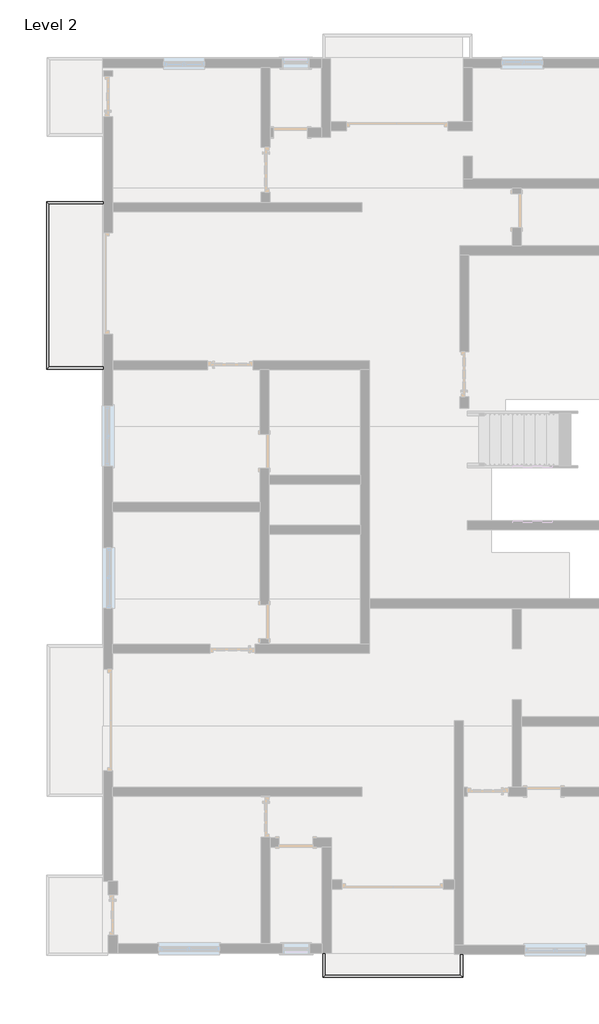
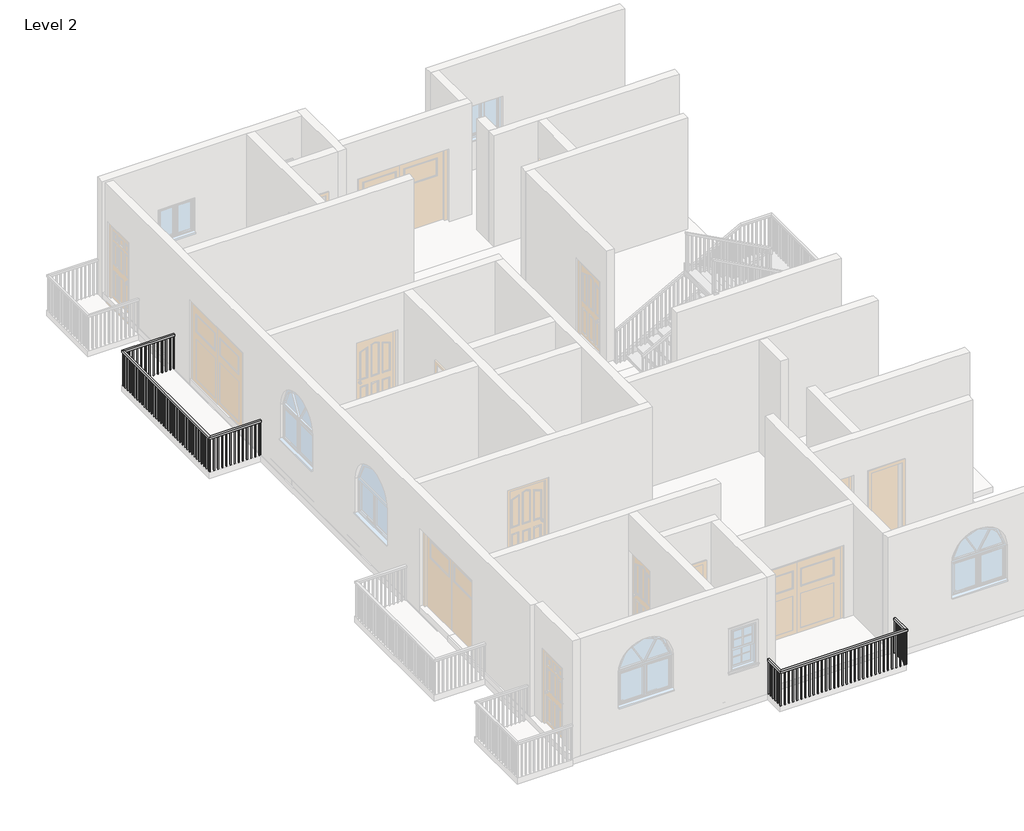
# One storey, part 4 of 7: 2 railings.
"""IFC4 building model written with IfcOpenShell, lengths in millimetres."""

from ifc_helpers import new_model, si_unit, frame, origin, place, context, project, spatial, polyline, outline, extrude, faceted_brep, element, save

model = new_model("IFC4")

# Units and contexts
model_context = context("Model", 3, world=origin())
ifc_project = project(units=[si_unit("LENGTHUNIT", "METRE", prefix="MILLI")], contexts=[model_context])

# Site, building, storey
site = spatial("IfcSite", under=ifc_project)
building = spatial("IfcBuilding", under=site)
storey = spatial("IfcBuildingStorey", under=building, Name="Level 2", Elevation=3048.0)

# Railings
placement = place(None, origin())
element("IfcRailing", 1, ObjectType="Handrail - Rectangular", at=placement, inside=storey, context=model_context, shape_type="SolidModel", body=[
    faceted_brep([(-1375.8109037, -10612.9037749, 3962.4), (-1375.8109037, -10612.9037749, 3911.6), (-1426.6109037, -10612.9037749, 3911.6), (-1426.6109037, -10612.9037749, 3962.4), (-1375.8109037, -11108.2037749, 3962.4), (-1375.8109037, -11108.2037749, 3911.6), (-1426.6109037, -11159.0037749, 3911.6), (-1426.6109037, -11159.0037749, 3962.4), (1659.4890963, -11108.2037749, 3962.4), (1659.4890963, -11108.2037749, 3911.6), (1710.2890963, -11159.0037749, 3911.6), (1710.2890963, -11159.0037749, 3962.4), (1659.4890963, -10638.3037749, 3962.4), (1710.2890963, -10638.3037749, 3962.4), (1710.2890963, -10638.3037749, 3911.6), (1659.4890963, -10638.3037749, 3911.6)], [[[0, 1, 2, 3]], [[1, 0, 4, 5]], [[2, 1, 5, 6]], [[3, 2, 6, 7]], [[0, 3, 7, 4]], [[5, 4, 8, 9]], [[6, 5, 9, 10]], [[7, 6, 10, 11]], [[4, 7, 11, 8]], [[12, 13, 14, 15]], [[9, 8, 12, 15]], [[10, 9, 15, 14]], [[11, 10, 14, 13]], [[8, 11, 13, 12]]]),
    extrude(outline(polyline([(1694.4140963, -10736.7287749), (1675.3640963, -10736.7287749), (1675.3640963, -10717.6787749), (1694.4140963, -10717.6787749), (1694.4140963, -10736.7287749)])), frame((0.0, 0.0, 3048.0), z_axis=(0.0, 0.0, 1.0), x_axis=(1.0, 0.0, 0.0)), (0.0, 0.0, 1.0), 863.6),
    extrude(outline(polyline([(1694.4140963, -10838.3287749), (1675.3640963, -10838.3287749), (1675.3640963, -10819.2787749), (1694.4140963, -10819.2787749), (1694.4140963, -10838.3287749)])), frame((0.0, 0.0, 3048.0), z_axis=(0.0, 0.0, 1.0), x_axis=(1.0, 0.0, 0.0)), (0.0, 0.0, 1.0), 863.6),
    extrude(outline(polyline([(1694.4140963, -10939.9287749), (1675.3640963, -10939.9287749), (1675.3640963, -10920.8787749), (1694.4140963, -10920.8787749), (1694.4140963, -10939.9287749)])), frame((0.0, 0.0, 3048.0), z_axis=(0.0, 0.0, 1.0), x_axis=(1.0, 0.0, 0.0)), (0.0, 0.0, 1.0), 863.6),
    extrude(outline(polyline([(1694.4140963, -11041.5287749), (1675.3640963, -11041.5287749), (1675.3640963, -11022.4787749), (1694.4140963, -11022.4787749), (1694.4140963, -11041.5287749)])), frame((0.0, 0.0, 3048.0), z_axis=(0.0, 0.0, 1.0), x_axis=(1.0, 0.0, 0.0)), (0.0, 0.0, 1.0), 863.6),
    extrude(outline(polyline([(1637.2640963, -11143.1287749), (1637.2640963, -11124.0787749), (1656.3140963, -11124.0787749), (1656.3140963, -11143.1287749), (1637.2640963, -11143.1287749)])), frame((0.0, 0.0, 3048.0), z_axis=(0.0, 0.0, 1.0), x_axis=(1.0, 0.0, 0.0)), (0.0, 0.0, 1.0), 863.6),
    extrude(outline(polyline([(1535.6640963, -11143.1287749), (1535.6640963, -11124.0787749), (1554.7140963, -11124.0787749), (1554.7140963, -11143.1287749), (1535.6640963, -11143.1287749)])), frame((0.0, 0.0, 3048.0), z_axis=(0.0, 0.0, 1.0), x_axis=(1.0, 0.0, 0.0)), (0.0, 0.0, 1.0), 863.6),
    extrude(outline(polyline([(1434.0640963, -11143.1287749), (1434.0640963, -11124.0787749), (1453.1140963, -11124.0787749), (1453.1140963, -11143.1287749), (1434.0640963, -11143.1287749)])), frame((0.0, 0.0, 3048.0), z_axis=(0.0, 0.0, 1.0), x_axis=(1.0, 0.0, 0.0)), (0.0, 0.0, 1.0), 863.6),
    extrude(outline(polyline([(1332.4640963, -11143.1287749), (1332.4640963, -11124.0787749), (1351.5140963, -11124.0787749), (1351.5140963, -11143.1287749), (1332.4640963, -11143.1287749)])), frame((0.0, 0.0, 3048.0), z_axis=(0.0, 0.0, 1.0), x_axis=(1.0, 0.0, 0.0)), (0.0, 0.0, 1.0), 863.6),
    extrude(outline(polyline([(1230.8640963, -11143.1287749), (1230.8640963, -11124.0787749), (1249.9140963, -11124.0787749), (1249.9140963, -11143.1287749), (1230.8640963, -11143.1287749)])), frame((0.0, 0.0, 3048.0), z_axis=(0.0, 0.0, 1.0), x_axis=(1.0, 0.0, 0.0)), (0.0, 0.0, 1.0), 863.6),
    extrude(outline(polyline([(1129.2640963, -11143.1287749), (1129.2640963, -11124.0787749), (1148.3140963, -11124.0787749), (1148.3140963, -11143.1287749), (1129.2640963, -11143.1287749)])), frame((0.0, 0.0, 3048.0), z_axis=(0.0, 0.0, 1.0), x_axis=(1.0, 0.0, 0.0)), (0.0, 0.0, 1.0), 863.6),
    extrude(outline(polyline([(1027.6640963, -11143.1287749), (1027.6640963, -11124.0787749), (1046.7140963, -11124.0787749), (1046.7140963, -11143.1287749), (1027.6640963, -11143.1287749)])), frame((0.0, 0.0, 3048.0), z_axis=(0.0, 0.0, 1.0), x_axis=(1.0, 0.0, 0.0)), (0.0, 0.0, 1.0), 863.6),
    extrude(outline(polyline([(926.0640963, -11143.1287749), (926.0640963, -11124.0787749), (945.1140963, -11124.0787749), (945.1140963, -11143.1287749), (926.0640963, -11143.1287749)])), frame((0.0, 0.0, 3048.0), z_axis=(0.0, 0.0, 1.0), x_axis=(1.0, 0.0, 0.0)), (0.0, 0.0, 1.0), 863.6),
    extrude(outline(polyline([(824.4640963, -11143.1287749), (824.4640963, -11124.0787749), (843.5140963, -11124.0787749), (843.5140963, -11143.1287749), (824.4640963, -11143.1287749)])), frame((0.0, 0.0, 3048.0), z_axis=(0.0, 0.0, 1.0), x_axis=(1.0, 0.0, 0.0)), (0.0, 0.0, 1.0), 863.6),
    extrude(outline(polyline([(722.8640963, -11143.1287749), (722.8640963, -11124.0787749), (741.9140963, -11124.0787749), (741.9140963, -11143.1287749), (722.8640963, -11143.1287749)])), frame((0.0, 0.0, 3048.0), z_axis=(0.0, 0.0, 1.0), x_axis=(1.0, 0.0, 0.0)), (0.0, 0.0, 1.0), 863.6),
    extrude(outline(polyline([(621.2640963, -11143.1287749), (621.2640963, -11124.0787749), (640.3140963, -11124.0787749), (640.3140963, -11143.1287749), (621.2640963, -11143.1287749)])), frame((0.0, 0.0, 3048.0), z_axis=(0.0, 0.0, 1.0), x_axis=(1.0, 0.0, 0.0)), (0.0, 0.0, 1.0), 863.6),
    extrude(outline(polyline([(519.6640963, -11143.1287749), (519.6640963, -11124.0787749), (538.7140963, -11124.0787749), (538.7140963, -11143.1287749), (519.6640963, -11143.1287749)])), frame((0.0, 0.0, 3048.0), z_axis=(0.0, 0.0, 1.0), x_axis=(1.0, 0.0, 0.0)), (0.0, 0.0, 1.0), 863.6),
    extrude(outline(polyline([(418.0640963, -11143.1287749), (418.0640963, -11124.0787749), (437.1140963, -11124.0787749), (437.1140963, -11143.1287749), (418.0640963, -11143.1287749)])), frame((0.0, 0.0, 3048.0), z_axis=(0.0, 0.0, 1.0), x_axis=(1.0, 0.0, 0.0)), (0.0, 0.0, 1.0), 863.6),
    extrude(outline(polyline([(316.4640963, -11143.1287749), (316.4640963, -11124.0787749), (335.5140963, -11124.0787749), (335.5140963, -11143.1287749), (316.4640963, -11143.1287749)])), frame((0.0, 0.0, 3048.0), z_axis=(0.0, 0.0, 1.0), x_axis=(1.0, 0.0, 0.0)), (0.0, 0.0, 1.0), 863.6),
    extrude(outline(polyline([(214.8640963, -11143.1287749), (214.8640963, -11124.0787749), (233.9140963, -11124.0787749), (233.9140963, -11143.1287749), (214.8640963, -11143.1287749)])), frame((0.0, 0.0, 3048.0), z_axis=(0.0, 0.0, 1.0), x_axis=(1.0, 0.0, 0.0)), (0.0, 0.0, 1.0), 863.6),
    extrude(outline(polyline([(113.2640963, -11143.1287749), (113.2640963, -11124.0787749), (132.3140963, -11124.0787749), (132.3140963, -11143.1287749), (113.2640963, -11143.1287749)])), frame((0.0, 0.0, 3048.0), z_axis=(0.0, 0.0, 1.0), x_axis=(1.0, 0.0, 0.0)), (0.0, 0.0, 1.0), 863.6),
    extrude(outline(polyline([(11.6640963, -11143.1287749), (11.6640963, -11124.0787749), (30.7140963, -11124.0787749), (30.7140963, -11143.1287749), (11.6640963, -11143.1287749)])), frame((0.0, 0.0, 3048.0), z_axis=(0.0, 0.0, 1.0), x_axis=(1.0, 0.0, 0.0)), (0.0, 0.0, 1.0), 863.6),
    extrude(outline(polyline([(-89.9359037, -11143.1287749), (-89.9359037, -11124.0787749), (-70.8859037, -11124.0787749), (-70.8859037, -11143.1287749), (-89.9359037, -11143.1287749)])), frame((0.0, 0.0, 3048.0), z_axis=(0.0, 0.0, 1.0), x_axis=(1.0, 0.0, 0.0)), (0.0, 0.0, 1.0), 863.6),
    extrude(outline(polyline([(-191.5359037, -11143.1287749), (-191.5359037, -11124.0787749), (-172.4859037, -11124.0787749), (-172.4859037, -11143.1287749), (-191.5359037, -11143.1287749)])), frame((0.0, 0.0, 3048.0), z_axis=(0.0, 0.0, 1.0), x_axis=(1.0, 0.0, 0.0)), (0.0, 0.0, 1.0), 863.6),
    extrude(outline(polyline([(-293.1359037, -11143.1287749), (-293.1359037, -11124.0787749), (-274.0859037, -11124.0787749), (-274.0859037, -11143.1287749), (-293.1359037, -11143.1287749)])), frame((0.0, 0.0, 3048.0), z_axis=(0.0, 0.0, 1.0), x_axis=(1.0, 0.0, 0.0)), (0.0, 0.0, 1.0), 863.6),
    extrude(outline(polyline([(-394.7359037, -11143.1287749), (-394.7359037, -11124.0787749), (-375.6859037, -11124.0787749), (-375.6859037, -11143.1287749), (-394.7359037, -11143.1287749)])), frame((0.0, 0.0, 3048.0), z_axis=(0.0, 0.0, 1.0), x_axis=(1.0, 0.0, 0.0)), (0.0, 0.0, 1.0), 863.6),
    extrude(outline(polyline([(-496.3359037, -11143.1287749), (-496.3359037, -11124.0787749), (-477.2859037, -11124.0787749), (-477.2859037, -11143.1287749), (-496.3359037, -11143.1287749)])), frame((0.0, 0.0, 3048.0), z_axis=(0.0, 0.0, 1.0), x_axis=(1.0, 0.0, 0.0)), (0.0, 0.0, 1.0), 863.6),
    extrude(outline(polyline([(-597.9359037, -11143.1287749), (-597.9359037, -11124.0787749), (-578.8859037, -11124.0787749), (-578.8859037, -11143.1287749), (-597.9359037, -11143.1287749)])), frame((0.0, 0.0, 3048.0), z_axis=(0.0, 0.0, 1.0), x_axis=(1.0, 0.0, 0.0)), (0.0, 0.0, 1.0), 863.6),
    extrude(outline(polyline([(-699.5359037, -11143.1287749), (-699.5359037, -11124.0787749), (-680.4859037, -11124.0787749), (-680.4859037, -11143.1287749), (-699.5359037, -11143.1287749)])), frame((0.0, 0.0, 3048.0), z_axis=(0.0, 0.0, 1.0), x_axis=(1.0, 0.0, 0.0)), (0.0, 0.0, 1.0), 863.6),
    extrude(outline(polyline([(-801.1359037, -11143.1287749), (-801.1359037, -11124.0787749), (-782.0859037, -11124.0787749), (-782.0859037, -11143.1287749), (-801.1359037, -11143.1287749)])), frame((0.0, 0.0, 3048.0), z_axis=(0.0, 0.0, 1.0), x_axis=(1.0, 0.0, 0.0)), (0.0, 0.0, 1.0), 863.6),
    extrude(outline(polyline([(-902.7359037, -11143.1287749), (-902.7359037, -11124.0787749), (-883.6859037, -11124.0787749), (-883.6859037, -11143.1287749), (-902.7359037, -11143.1287749)])), frame((0.0, 0.0, 3048.0), z_axis=(0.0, 0.0, 1.0), x_axis=(1.0, 0.0, 0.0)), (0.0, 0.0, 1.0), 863.6),
    extrude(outline(polyline([(-1004.3359037, -11143.1287749), (-1004.3359037, -11124.0787749), (-985.2859037, -11124.0787749), (-985.2859037, -11143.1287749), (-1004.3359037, -11143.1287749)])), frame((0.0, 0.0, 3048.0), z_axis=(0.0, 0.0, 1.0), x_axis=(1.0, 0.0, 0.0)), (0.0, 0.0, 1.0), 863.6),
    extrude(outline(polyline([(-1105.9359037, -11143.1287749), (-1105.9359037, -11124.0787749), (-1086.8859037, -11124.0787749), (-1086.8859037, -11143.1287749), (-1105.9359037, -11143.1287749)])), frame((0.0, 0.0, 3048.0), z_axis=(0.0, 0.0, 1.0), x_axis=(1.0, 0.0, 0.0)), (0.0, 0.0, 1.0), 863.6),
    extrude(outline(polyline([(-1207.5359037, -11143.1287749), (-1207.5359037, -11124.0787749), (-1188.4859037, -11124.0787749), (-1188.4859037, -11143.1287749), (-1207.5359037, -11143.1287749)])), frame((0.0, 0.0, 3048.0), z_axis=(0.0, 0.0, 1.0), x_axis=(1.0, 0.0, 0.0)), (0.0, 0.0, 1.0), 863.6),
    extrude(outline(polyline([(-1309.1359037, -11143.1287749), (-1309.1359037, -11124.0787749), (-1290.0859037, -11124.0787749), (-1290.0859037, -11143.1287749), (-1309.1359037, -11143.1287749)])), frame((0.0, 0.0, 3048.0), z_axis=(0.0, 0.0, 1.0), x_axis=(1.0, 0.0, 0.0)), (0.0, 0.0, 1.0), 863.6),
    extrude(outline(polyline([(-1410.7359037, -11111.3787749), (-1391.6859037, -11111.3787749), (-1391.6859037, -11130.4287749), (-1410.7359037, -11130.4287749), (-1410.7359037, -11111.3787749)])), frame((0.0, 0.0, 3048.0), z_axis=(0.0, 0.0, 1.0), x_axis=(1.0, 0.0, 0.0)), (0.0, 0.0, 1.0), 863.6),
    extrude(outline(polyline([(-1410.7359037, -11009.7787749), (-1391.6859037, -11009.7787749), (-1391.6859037, -11028.8287749), (-1410.7359037, -11028.8287749), (-1410.7359037, -11009.7787749)])), frame((0.0, 0.0, 3048.0), z_axis=(0.0, 0.0, 1.0), x_axis=(1.0, 0.0, 0.0)), (0.0, 0.0, 1.0), 863.6),
    extrude(outline(polyline([(-1410.7359037, -10908.1787749), (-1391.6859037, -10908.1787749), (-1391.6859037, -10927.2287749), (-1410.7359037, -10927.2287749), (-1410.7359037, -10908.1787749)])), frame((0.0, 0.0, 3048.0), z_axis=(0.0, 0.0, 1.0), x_axis=(1.0, 0.0, 0.0)), (0.0, 0.0, 1.0), 863.6),
    extrude(outline(polyline([(-1410.7359037, -10806.5787749), (-1391.6859037, -10806.5787749), (-1391.6859037, -10825.6287749), (-1410.7359037, -10825.6287749), (-1410.7359037, -10806.5787749)])), frame((0.0, 0.0, 3048.0), z_axis=(0.0, 0.0, 1.0), x_axis=(1.0, 0.0, 0.0)), (0.0, 0.0, 1.0), 863.6),
    extrude(outline(polyline([(-1410.7359037, -10704.9787749), (-1391.6859037, -10704.9787749), (-1391.6859037, -10724.0287749), (-1410.7359037, -10724.0287749), (-1410.7359037, -10704.9787749)])), frame((0.0, 0.0, 3048.0), z_axis=(0.0, 0.0, 1.0), x_axis=(1.0, 0.0, 0.0)), (0.0, 0.0, 1.0), 863.6),
    extrude(outline(polyline([(1675.3640963, -11143.1287749), (1675.3640963, -11124.0787749), (1694.4140963, -11124.0787749), (1694.4140963, -11143.1287749), (1675.3640963, -11143.1287749)])), frame((0.0, 0.0, 3048.0), z_axis=(0.0, 0.0, 1.0), x_axis=(1.0, 0.0, 0.0)), (0.0, 0.0, 1.0), 863.6),
    extrude(outline(polyline([(-1410.7359037, -11124.0787749), (-1391.6859037, -11124.0787749), (-1391.6859037, -11143.1287749), (-1410.7359037, -11143.1287749), (-1410.7359037, -11124.0787749)])), frame((0.0, 0.0, 3048.0), z_axis=(0.0, 0.0, 1.0), x_axis=(1.0, 0.0, 0.0)), (0.0, 0.0, 1.0), 863.6),
    extrude(outline(polyline([(1694.4140963, -10657.3537749), (1675.3640963, -10657.3537749), (1675.3640963, -10638.3037749), (1694.4140963, -10638.3037749), (1694.4140963, -10657.3537749)])), frame((0.0, 0.0, 3048.0), z_axis=(0.0, 0.0, 1.0), x_axis=(1.0, 0.0, 0.0)), (0.0, 0.0, 1.0), 863.6),
    extrude(outline(polyline([(-1410.7359037, -10612.9037749), (-1391.6859037, -10612.9037749), (-1391.6859037, -10631.9537749), (-1410.7359037, -10631.9537749), (-1410.7359037, -10612.9037749)])), frame((0.0, 0.0, 3048.0), z_axis=(0.0, 0.0, 1.0), x_axis=(1.0, 0.0, 0.0)), (0.0, 0.0, 1.0), 863.6),
])
element("IfcRailing", 2, ObjectType="Handrail - Rectangular", at=placement, inside=storey, context=model_context, shape_type="SolidModel", body=[
    faceted_brep([(-6330.8013636, 6151.0962251, 3962.4), (-6330.8013636, 6151.0962251, 3911.6), (-6330.8013636, 6201.8962251, 3911.6), (-6330.8013636, 6201.8962251, 3962.4), (-7563.8859037, 6151.0962251, 3962.4), (-7563.8859037, 6151.0962251, 3911.6), (-7614.6859037, 6201.8962251, 3911.6), (-7614.6859037, 6201.8962251, 3962.4), (-7563.8859037, 2506.1962251, 3962.4), (-7563.8859037, 2506.1962251, 3911.6), (-7614.6859037, 2455.3962251, 3911.6), (-7614.6859037, 2455.3962251, 3962.4), (-6330.8013636, 2506.1962251, 3962.4), (-6330.8013636, 2455.3962251, 3962.4), (-6330.8013636, 2455.3962251, 3911.6), (-6330.8013636, 2506.1962251, 3911.6)], [[[0, 1, 2, 3]], [[1, 0, 4, 5]], [[2, 1, 5, 6]], [[3, 2, 6, 7]], [[0, 3, 7, 4]], [[5, 4, 8, 9]], [[6, 5, 9, 10]], [[7, 6, 10, 11]], [[4, 7, 11, 8]], [[12, 13, 14, 15]], [[9, 8, 12, 15]], [[10, 9, 15, 14]], [[11, 10, 14, 13]], [[8, 11, 13, 12]]]),
    extrude(outline(polyline([(-6379.6109037, 2471.2712251), (-6379.6109037, 2490.3212251), (-6360.5609037, 2490.3212251), (-6360.5609037, 2471.2712251), (-6379.6109037, 2471.2712251)])), frame((0.0, 0.0, 3048.0), z_axis=(0.0, 0.0, 1.0), x_axis=(1.0, 0.0, 0.0)), (0.0, 0.0, 1.0), 863.6),
    extrude(outline(polyline([(-6481.2109037, 2471.2712251), (-6481.2109037, 2490.3212251), (-6462.1609037, 2490.3212251), (-6462.1609037, 2471.2712251), (-6481.2109037, 2471.2712251)])), frame((0.0, 0.0, 3048.0), z_axis=(0.0, 0.0, 1.0), x_axis=(1.0, 0.0, 0.0)), (0.0, 0.0, 1.0), 863.6),
    extrude(outline(polyline([(-6582.8109037, 2471.2712251), (-6582.8109037, 2490.3212251), (-6563.7609037, 2490.3212251), (-6563.7609037, 2471.2712251), (-6582.8109037, 2471.2712251)])), frame((0.0, 0.0, 3048.0), z_axis=(0.0, 0.0, 1.0), x_axis=(1.0, 0.0, 0.0)), (0.0, 0.0, 1.0), 863.6),
    extrude(outline(polyline([(-6684.4109037, 2471.2712251), (-6684.4109037, 2490.3212251), (-6665.3609037, 2490.3212251), (-6665.3609037, 2471.2712251), (-6684.4109037, 2471.2712251)])), frame((0.0, 0.0, 3048.0), z_axis=(0.0, 0.0, 1.0), x_axis=(1.0, 0.0, 0.0)), (0.0, 0.0, 1.0), 863.6),
    extrude(outline(polyline([(-6786.0109037, 2471.2712251), (-6786.0109037, 2490.3212251), (-6766.9609037, 2490.3212251), (-6766.9609037, 2471.2712251), (-6786.0109037, 2471.2712251)])), frame((0.0, 0.0, 3048.0), z_axis=(0.0, 0.0, 1.0), x_axis=(1.0, 0.0, 0.0)), (0.0, 0.0, 1.0), 863.6),
    extrude(outline(polyline([(-6887.6109037, 2471.2712251), (-6887.6109037, 2490.3212251), (-6868.5609037, 2490.3212251), (-6868.5609037, 2471.2712251), (-6887.6109037, 2471.2712251)])), frame((0.0, 0.0, 3048.0), z_axis=(0.0, 0.0, 1.0), x_axis=(1.0, 0.0, 0.0)), (0.0, 0.0, 1.0), 863.6),
    extrude(outline(polyline([(-6989.2109037, 2471.2712251), (-6989.2109037, 2490.3212251), (-6970.1609037, 2490.3212251), (-6970.1609037, 2471.2712251), (-6989.2109037, 2471.2712251)])), frame((0.0, 0.0, 3048.0), z_axis=(0.0, 0.0, 1.0), x_axis=(1.0, 0.0, 0.0)), (0.0, 0.0, 1.0), 863.6),
    extrude(outline(polyline([(-7090.8109037, 2471.2712251), (-7090.8109037, 2490.3212251), (-7071.7609037, 2490.3212251), (-7071.7609037, 2471.2712251), (-7090.8109037, 2471.2712251)])), frame((0.0, 0.0, 3048.0), z_axis=(0.0, 0.0, 1.0), x_axis=(1.0, 0.0, 0.0)), (0.0, 0.0, 1.0), 863.6),
    extrude(outline(polyline([(-7192.4109037, 2471.2712251), (-7192.4109037, 2490.3212251), (-7173.3609037, 2490.3212251), (-7173.3609037, 2471.2712251), (-7192.4109037, 2471.2712251)])), frame((0.0, 0.0, 3048.0), z_axis=(0.0, 0.0, 1.0), x_axis=(1.0, 0.0, 0.0)), (0.0, 0.0, 1.0), 863.6),
    extrude(outline(polyline([(-7294.0109037, 2471.2712251), (-7294.0109037, 2490.3212251), (-7274.9609037, 2490.3212251), (-7274.9609037, 2471.2712251), (-7294.0109037, 2471.2712251)])), frame((0.0, 0.0, 3048.0), z_axis=(0.0, 0.0, 1.0), x_axis=(1.0, 0.0, 0.0)), (0.0, 0.0, 1.0), 863.6),
    extrude(outline(polyline([(-7395.6109037, 2471.2712251), (-7395.6109037, 2490.3212251), (-7376.5609037, 2490.3212251), (-7376.5609037, 2471.2712251), (-7395.6109037, 2471.2712251)])), frame((0.0, 0.0, 3048.0), z_axis=(0.0, 0.0, 1.0), x_axis=(1.0, 0.0, 0.0)), (0.0, 0.0, 1.0), 863.6),
    extrude(outline(polyline([(-7497.2109037, 2471.2712251), (-7497.2109037, 2490.3212251), (-7478.1609037, 2490.3212251), (-7478.1609037, 2471.2712251), (-7497.2109037, 2471.2712251)])), frame((0.0, 0.0, 3048.0), z_axis=(0.0, 0.0, 1.0), x_axis=(1.0, 0.0, 0.0)), (0.0, 0.0, 1.0), 863.6),
    extrude(outline(polyline([(-7598.8109037, 2528.4212251), (-7579.7609037, 2528.4212251), (-7579.7609037, 2509.3712251), (-7598.8109037, 2509.3712251), (-7598.8109037, 2528.4212251)])), frame((0.0, 0.0, 3048.0), z_axis=(0.0, 0.0, 1.0), x_axis=(1.0, 0.0, 0.0)), (0.0, 0.0, 1.0), 863.6),
    extrude(outline(polyline([(-7598.8109037, 2630.0212251), (-7579.7609037, 2630.0212251), (-7579.7609037, 2610.9712251), (-7598.8109037, 2610.9712251), (-7598.8109037, 2630.0212251)])), frame((0.0, 0.0, 3048.0), z_axis=(0.0, 0.0, 1.0), x_axis=(1.0, 0.0, 0.0)), (0.0, 0.0, 1.0), 863.6),
    extrude(outline(polyline([(-7598.8109037, 2731.6212251), (-7579.7609037, 2731.6212251), (-7579.7609037, 2712.5712251), (-7598.8109037, 2712.5712251), (-7598.8109037, 2731.6212251)])), frame((0.0, 0.0, 3048.0), z_axis=(0.0, 0.0, 1.0), x_axis=(1.0, 0.0, 0.0)), (0.0, 0.0, 1.0), 863.6),
    extrude(outline(polyline([(-7598.8109037, 2833.2212251), (-7579.7609037, 2833.2212251), (-7579.7609037, 2814.1712251), (-7598.8109037, 2814.1712251), (-7598.8109037, 2833.2212251)])), frame((0.0, 0.0, 3048.0), z_axis=(0.0, 0.0, 1.0), x_axis=(1.0, 0.0, 0.0)), (0.0, 0.0, 1.0), 863.6),
    extrude(outline(polyline([(-7598.8109037, 2934.8212251), (-7579.7609037, 2934.8212251), (-7579.7609037, 2915.7712251), (-7598.8109037, 2915.7712251), (-7598.8109037, 2934.8212251)])), frame((0.0, 0.0, 3048.0), z_axis=(0.0, 0.0, 1.0), x_axis=(1.0, 0.0, 0.0)), (0.0, 0.0, 1.0), 863.6),
    extrude(outline(polyline([(-7598.8109037, 3036.4212251), (-7579.7609037, 3036.4212251), (-7579.7609037, 3017.3712251), (-7598.8109037, 3017.3712251), (-7598.8109037, 3036.4212251)])), frame((0.0, 0.0, 3048.0), z_axis=(0.0, 0.0, 1.0), x_axis=(1.0, 0.0, 0.0)), (0.0, 0.0, 1.0), 863.6),
    extrude(outline(polyline([(-7598.8109037, 3138.0212251), (-7579.7609037, 3138.0212251), (-7579.7609037, 3118.9712251), (-7598.8109037, 3118.9712251), (-7598.8109037, 3138.0212251)])), frame((0.0, 0.0, 3048.0), z_axis=(0.0, 0.0, 1.0), x_axis=(1.0, 0.0, 0.0)), (0.0, 0.0, 1.0), 863.6),
    extrude(outline(polyline([(-7598.8109037, 3239.6212251), (-7579.7609037, 3239.6212251), (-7579.7609037, 3220.5712251), (-7598.8109037, 3220.5712251), (-7598.8109037, 3239.6212251)])), frame((0.0, 0.0, 3048.0), z_axis=(0.0, 0.0, 1.0), x_axis=(1.0, 0.0, 0.0)), (0.0, 0.0, 1.0), 863.6),
    extrude(outline(polyline([(-7598.8109037, 3341.2212251), (-7579.7609037, 3341.2212251), (-7579.7609037, 3322.1712251), (-7598.8109037, 3322.1712251), (-7598.8109037, 3341.2212251)])), frame((0.0, 0.0, 3048.0), z_axis=(0.0, 0.0, 1.0), x_axis=(1.0, 0.0, 0.0)), (0.0, 0.0, 1.0), 863.6),
    extrude(outline(polyline([(-7598.8109037, 3442.8212251), (-7579.7609037, 3442.8212251), (-7579.7609037, 3423.7712251), (-7598.8109037, 3423.7712251), (-7598.8109037, 3442.8212251)])), frame((0.0, 0.0, 3048.0), z_axis=(0.0, 0.0, 1.0), x_axis=(1.0, 0.0, 0.0)), (0.0, 0.0, 1.0), 863.6),
    extrude(outline(polyline([(-7598.8109037, 3544.4212251), (-7579.7609037, 3544.4212251), (-7579.7609037, 3525.3712251), (-7598.8109037, 3525.3712251), (-7598.8109037, 3544.4212251)])), frame((0.0, 0.0, 3048.0), z_axis=(0.0, 0.0, 1.0), x_axis=(1.0, 0.0, 0.0)), (0.0, 0.0, 1.0), 863.6),
    extrude(outline(polyline([(-7598.8109037, 3646.0212251), (-7579.7609037, 3646.0212251), (-7579.7609037, 3626.9712251), (-7598.8109037, 3626.9712251), (-7598.8109037, 3646.0212251)])), frame((0.0, 0.0, 3048.0), z_axis=(0.0, 0.0, 1.0), x_axis=(1.0, 0.0, 0.0)), (0.0, 0.0, 1.0), 863.6),
    extrude(outline(polyline([(-7598.8109037, 3747.6212251), (-7579.7609037, 3747.6212251), (-7579.7609037, 3728.5712251), (-7598.8109037, 3728.5712251), (-7598.8109037, 3747.6212251)])), frame((0.0, 0.0, 3048.0), z_axis=(0.0, 0.0, 1.0), x_axis=(1.0, 0.0, 0.0)), (0.0, 0.0, 1.0), 863.6),
    extrude(outline(polyline([(-7598.8109037, 3849.2212251), (-7579.7609037, 3849.2212251), (-7579.7609037, 3830.1712251), (-7598.8109037, 3830.1712251), (-7598.8109037, 3849.2212251)])), frame((0.0, 0.0, 3048.0), z_axis=(0.0, 0.0, 1.0), x_axis=(1.0, 0.0, 0.0)), (0.0, 0.0, 1.0), 863.6),
    extrude(outline(polyline([(-7598.8109037, 3950.8212251), (-7579.7609037, 3950.8212251), (-7579.7609037, 3931.7712251), (-7598.8109037, 3931.7712251), (-7598.8109037, 3950.8212251)])), frame((0.0, 0.0, 3048.0), z_axis=(0.0, 0.0, 1.0), x_axis=(1.0, 0.0, 0.0)), (0.0, 0.0, 1.0), 863.6),
    extrude(outline(polyline([(-7598.8109037, 4052.4212251), (-7579.7609037, 4052.4212251), (-7579.7609037, 4033.3712251), (-7598.8109037, 4033.3712251), (-7598.8109037, 4052.4212251)])), frame((0.0, 0.0, 3048.0), z_axis=(0.0, 0.0, 1.0), x_axis=(1.0, 0.0, 0.0)), (0.0, 0.0, 1.0), 863.6),
    extrude(outline(polyline([(-7598.8109037, 4154.0212251), (-7579.7609037, 4154.0212251), (-7579.7609037, 4134.9712251), (-7598.8109037, 4134.9712251), (-7598.8109037, 4154.0212251)])), frame((0.0, 0.0, 3048.0), z_axis=(0.0, 0.0, 1.0), x_axis=(1.0, 0.0, 0.0)), (0.0, 0.0, 1.0), 863.6),
    extrude(outline(polyline([(-7598.8109037, 4255.6212251), (-7579.7609037, 4255.6212251), (-7579.7609037, 4236.5712251), (-7598.8109037, 4236.5712251), (-7598.8109037, 4255.6212251)])), frame((0.0, 0.0, 3048.0), z_axis=(0.0, 0.0, 1.0), x_axis=(1.0, 0.0, 0.0)), (0.0, 0.0, 1.0), 863.6),
    extrude(outline(polyline([(-7598.8109037, 4357.2212251), (-7579.7609037, 4357.2212251), (-7579.7609037, 4338.1712251), (-7598.8109037, 4338.1712251), (-7598.8109037, 4357.2212251)])), frame((0.0, 0.0, 3048.0), z_axis=(0.0, 0.0, 1.0), x_axis=(1.0, 0.0, 0.0)), (0.0, 0.0, 1.0), 863.6),
    extrude(outline(polyline([(-7598.8109037, 4458.8212251), (-7579.7609037, 4458.8212251), (-7579.7609037, 4439.7712251), (-7598.8109037, 4439.7712251), (-7598.8109037, 4458.8212251)])), frame((0.0, 0.0, 3048.0), z_axis=(0.0, 0.0, 1.0), x_axis=(1.0, 0.0, 0.0)), (0.0, 0.0, 1.0), 863.6),
    extrude(outline(polyline([(-7598.8109037, 4560.4212251), (-7579.7609037, 4560.4212251), (-7579.7609037, 4541.3712251), (-7598.8109037, 4541.3712251), (-7598.8109037, 4560.4212251)])), frame((0.0, 0.0, 3048.0), z_axis=(0.0, 0.0, 1.0), x_axis=(1.0, 0.0, 0.0)), (0.0, 0.0, 1.0), 863.6),
    extrude(outline(polyline([(-7598.8109037, 4662.0212251), (-7579.7609037, 4662.0212251), (-7579.7609037, 4642.9712251), (-7598.8109037, 4642.9712251), (-7598.8109037, 4662.0212251)])), frame((0.0, 0.0, 3048.0), z_axis=(0.0, 0.0, 1.0), x_axis=(1.0, 0.0, 0.0)), (0.0, 0.0, 1.0), 863.6),
    extrude(outline(polyline([(-7598.8109037, 4763.6212251), (-7579.7609037, 4763.6212251), (-7579.7609037, 4744.5712251), (-7598.8109037, 4744.5712251), (-7598.8109037, 4763.6212251)])), frame((0.0, 0.0, 3048.0), z_axis=(0.0, 0.0, 1.0), x_axis=(1.0, 0.0, 0.0)), (0.0, 0.0, 1.0), 863.6),
    extrude(outline(polyline([(-7598.8109037, 4865.2212251), (-7579.7609037, 4865.2212251), (-7579.7609037, 4846.1712251), (-7598.8109037, 4846.1712251), (-7598.8109037, 4865.2212251)])), frame((0.0, 0.0, 3048.0), z_axis=(0.0, 0.0, 1.0), x_axis=(1.0, 0.0, 0.0)), (0.0, 0.0, 1.0), 863.6),
    extrude(outline(polyline([(-7598.8109037, 4966.8212251), (-7579.7609037, 4966.8212251), (-7579.7609037, 4947.7712251), (-7598.8109037, 4947.7712251), (-7598.8109037, 4966.8212251)])), frame((0.0, 0.0, 3048.0), z_axis=(0.0, 0.0, 1.0), x_axis=(1.0, 0.0, 0.0)), (0.0, 0.0, 1.0), 863.6),
    extrude(outline(polyline([(-7598.8109037, 5068.4212251), (-7579.7609037, 5068.4212251), (-7579.7609037, 5049.3712251), (-7598.8109037, 5049.3712251), (-7598.8109037, 5068.4212251)])), frame((0.0, 0.0, 3048.0), z_axis=(0.0, 0.0, 1.0), x_axis=(1.0, 0.0, 0.0)), (0.0, 0.0, 1.0), 863.6),
    extrude(outline(polyline([(-7598.8109037, 5170.0212251), (-7579.7609037, 5170.0212251), (-7579.7609037, 5150.9712251), (-7598.8109037, 5150.9712251), (-7598.8109037, 5170.0212251)])), frame((0.0, 0.0, 3048.0), z_axis=(0.0, 0.0, 1.0), x_axis=(1.0, 0.0, 0.0)), (0.0, 0.0, 1.0), 863.6),
    extrude(outline(polyline([(-7598.8109037, 5271.6212251), (-7579.7609037, 5271.6212251), (-7579.7609037, 5252.5712251), (-7598.8109037, 5252.5712251), (-7598.8109037, 5271.6212251)])), frame((0.0, 0.0, 3048.0), z_axis=(0.0, 0.0, 1.0), x_axis=(1.0, 0.0, 0.0)), (0.0, 0.0, 1.0), 863.6),
    extrude(outline(polyline([(-7598.8109037, 5373.2212251), (-7579.7609037, 5373.2212251), (-7579.7609037, 5354.1712251), (-7598.8109037, 5354.1712251), (-7598.8109037, 5373.2212251)])), frame((0.0, 0.0, 3048.0), z_axis=(0.0, 0.0, 1.0), x_axis=(1.0, 0.0, 0.0)), (0.0, 0.0, 1.0), 863.6),
    extrude(outline(polyline([(-7598.8109037, 5474.8212251), (-7579.7609037, 5474.8212251), (-7579.7609037, 5455.7712251), (-7598.8109037, 5455.7712251), (-7598.8109037, 5474.8212251)])), frame((0.0, 0.0, 3048.0), z_axis=(0.0, 0.0, 1.0), x_axis=(1.0, 0.0, 0.0)), (0.0, 0.0, 1.0), 863.6),
    extrude(outline(polyline([(-7598.8109037, 5576.4212251), (-7579.7609037, 5576.4212251), (-7579.7609037, 5557.3712251), (-7598.8109037, 5557.3712251), (-7598.8109037, 5576.4212251)])), frame((0.0, 0.0, 3048.0), z_axis=(0.0, 0.0, 1.0), x_axis=(1.0, 0.0, 0.0)), (0.0, 0.0, 1.0), 863.6),
    extrude(outline(polyline([(-7598.8109037, 5678.0212251), (-7579.7609037, 5678.0212251), (-7579.7609037, 5658.9712251), (-7598.8109037, 5658.9712251), (-7598.8109037, 5678.0212251)])), frame((0.0, 0.0, 3048.0), z_axis=(0.0, 0.0, 1.0), x_axis=(1.0, 0.0, 0.0)), (0.0, 0.0, 1.0), 863.6),
    extrude(outline(polyline([(-7598.8109037, 5779.6212251), (-7579.7609037, 5779.6212251), (-7579.7609037, 5760.5712251), (-7598.8109037, 5760.5712251), (-7598.8109037, 5779.6212251)])), frame((0.0, 0.0, 3048.0), z_axis=(0.0, 0.0, 1.0), x_axis=(1.0, 0.0, 0.0)), (0.0, 0.0, 1.0), 863.6),
    extrude(outline(polyline([(-7598.8109037, 5881.2212251), (-7579.7609037, 5881.2212251), (-7579.7609037, 5862.1712251), (-7598.8109037, 5862.1712251), (-7598.8109037, 5881.2212251)])), frame((0.0, 0.0, 3048.0), z_axis=(0.0, 0.0, 1.0), x_axis=(1.0, 0.0, 0.0)), (0.0, 0.0, 1.0), 863.6),
    extrude(outline(polyline([(-7598.8109037, 5982.8212251), (-7579.7609037, 5982.8212251), (-7579.7609037, 5963.7712251), (-7598.8109037, 5963.7712251), (-7598.8109037, 5982.8212251)])), frame((0.0, 0.0, 3048.0), z_axis=(0.0, 0.0, 1.0), x_axis=(1.0, 0.0, 0.0)), (0.0, 0.0, 1.0), 863.6),
    extrude(outline(polyline([(-7598.8109037, 6084.4212251), (-7579.7609037, 6084.4212251), (-7579.7609037, 6065.3712251), (-7598.8109037, 6065.3712251), (-7598.8109037, 6084.4212251)])), frame((0.0, 0.0, 3048.0), z_axis=(0.0, 0.0, 1.0), x_axis=(1.0, 0.0, 0.0)), (0.0, 0.0, 1.0), 863.6),
    extrude(outline(polyline([(-7540.4763636, 6186.0212251), (-7540.4763636, 6166.9712251), (-7559.5263636, 6166.9712251), (-7559.5263636, 6186.0212251), (-7540.4763636, 6186.0212251)])), frame((0.0, 0.0, 3048.0), z_axis=(0.0, 0.0, 1.0), x_axis=(1.0, 0.0, 0.0)), (0.0, 0.0, 1.0), 863.6),
    extrude(outline(polyline([(-7438.8763636, 6186.0212251), (-7438.8763636, 6166.9712251), (-7457.9263636, 6166.9712251), (-7457.9263636, 6186.0212251), (-7438.8763636, 6186.0212251)])), frame((0.0, 0.0, 3048.0), z_axis=(0.0, 0.0, 1.0), x_axis=(1.0, 0.0, 0.0)), (0.0, 0.0, 1.0), 863.6),
    extrude(outline(polyline([(-7337.2763636, 6186.0212251), (-7337.2763636, 6166.9712251), (-7356.3263636, 6166.9712251), (-7356.3263636, 6186.0212251), (-7337.2763636, 6186.0212251)])), frame((0.0, 0.0, 3048.0), z_axis=(0.0, 0.0, 1.0), x_axis=(1.0, 0.0, 0.0)), (0.0, 0.0, 1.0), 863.6),
    extrude(outline(polyline([(-7235.6763636, 6186.0212251), (-7235.6763636, 6166.9712251), (-7254.7263636, 6166.9712251), (-7254.7263636, 6186.0212251), (-7235.6763636, 6186.0212251)])), frame((0.0, 0.0, 3048.0), z_axis=(0.0, 0.0, 1.0), x_axis=(1.0, 0.0, 0.0)), (0.0, 0.0, 1.0), 863.6),
    extrude(outline(polyline([(-7134.0763636, 6186.0212251), (-7134.0763636, 6166.9712251), (-7153.1263636, 6166.9712251), (-7153.1263636, 6186.0212251), (-7134.0763636, 6186.0212251)])), frame((0.0, 0.0, 3048.0), z_axis=(0.0, 0.0, 1.0), x_axis=(1.0, 0.0, 0.0)), (0.0, 0.0, 1.0), 863.6),
    extrude(outline(polyline([(-7032.4763636, 6186.0212251), (-7032.4763636, 6166.9712251), (-7051.5263636, 6166.9712251), (-7051.5263636, 6186.0212251), (-7032.4763636, 6186.0212251)])), frame((0.0, 0.0, 3048.0), z_axis=(0.0, 0.0, 1.0), x_axis=(1.0, 0.0, 0.0)), (0.0, 0.0, 1.0), 863.6),
    extrude(outline(polyline([(-6930.8763636, 6186.0212251), (-6930.8763636, 6166.9712251), (-6949.9263636, 6166.9712251), (-6949.9263636, 6186.0212251), (-6930.8763636, 6186.0212251)])), frame((0.0, 0.0, 3048.0), z_axis=(0.0, 0.0, 1.0), x_axis=(1.0, 0.0, 0.0)), (0.0, 0.0, 1.0), 863.6),
    extrude(outline(polyline([(-6829.2763636, 6186.0212251), (-6829.2763636, 6166.9712251), (-6848.3263636, 6166.9712251), (-6848.3263636, 6186.0212251), (-6829.2763636, 6186.0212251)])), frame((0.0, 0.0, 3048.0), z_axis=(0.0, 0.0, 1.0), x_axis=(1.0, 0.0, 0.0)), (0.0, 0.0, 1.0), 863.6),
    extrude(outline(polyline([(-6727.6763636, 6186.0212251), (-6727.6763636, 6166.9712251), (-6746.7263636, 6166.9712251), (-6746.7263636, 6186.0212251), (-6727.6763636, 6186.0212251)])), frame((0.0, 0.0, 3048.0), z_axis=(0.0, 0.0, 1.0), x_axis=(1.0, 0.0, 0.0)), (0.0, 0.0, 1.0), 863.6),
    extrude(outline(polyline([(-6626.0763636, 6186.0212251), (-6626.0763636, 6166.9712251), (-6645.1263636, 6166.9712251), (-6645.1263636, 6186.0212251), (-6626.0763636, 6186.0212251)])), frame((0.0, 0.0, 3048.0), z_axis=(0.0, 0.0, 1.0), x_axis=(1.0, 0.0, 0.0)), (0.0, 0.0, 1.0), 863.6),
    extrude(outline(polyline([(-6524.4763636, 6186.0212251), (-6524.4763636, 6166.9712251), (-6543.5263636, 6166.9712251), (-6543.5263636, 6186.0212251), (-6524.4763636, 6186.0212251)])), frame((0.0, 0.0, 3048.0), z_axis=(0.0, 0.0, 1.0), x_axis=(1.0, 0.0, 0.0)), (0.0, 0.0, 1.0), 863.6),
    extrude(outline(polyline([(-6422.8763636, 6186.0212251), (-6422.8763636, 6166.9712251), (-6441.9263636, 6166.9712251), (-6441.9263636, 6186.0212251), (-6422.8763636, 6186.0212251)])), frame((0.0, 0.0, 3048.0), z_axis=(0.0, 0.0, 1.0), x_axis=(1.0, 0.0, 0.0)), (0.0, 0.0, 1.0), 863.6),
    extrude(outline(polyline([(-7598.8109037, 2490.3212251), (-7579.7609037, 2490.3212251), (-7579.7609037, 2471.2712251), (-7598.8109037, 2471.2712251), (-7598.8109037, 2490.3212251)])), frame((0.0, 0.0, 3048.0), z_axis=(0.0, 0.0, 1.0), x_axis=(1.0, 0.0, 0.0)), (0.0, 0.0, 1.0), 863.6),
    extrude(outline(polyline([(-7579.7609037, 6186.0212251), (-7579.7609037, 6166.9712251), (-7598.8109037, 6166.9712251), (-7598.8109037, 6186.0212251), (-7579.7609037, 6186.0212251)])), frame((0.0, 0.0, 3048.0), z_axis=(0.0, 0.0, 1.0), x_axis=(1.0, 0.0, 0.0)), (0.0, 0.0, 1.0), 863.6),
    extrude(outline(polyline([(-6349.8513636, 2471.2712251), (-6349.8513636, 2490.3212251), (-6330.8013636, 2490.3212251), (-6330.8013636, 2471.2712251), (-6349.8513636, 2471.2712251)])), frame((0.0, 0.0, 3048.0), z_axis=(0.0, 0.0, 1.0), x_axis=(1.0, 0.0, 0.0)), (0.0, 0.0, 1.0), 863.6),
    extrude(outline(polyline([(-6330.8013636, 6186.0212251), (-6330.8013636, 6166.9712251), (-6349.8513636, 6166.9712251), (-6349.8513636, 6186.0212251), (-6330.8013636, 6186.0212251)])), frame((0.0, 0.0, 3048.0), z_axis=(0.0, 0.0, 1.0), x_axis=(1.0, 0.0, 0.0)), (0.0, 0.0, 1.0), 863.6),
])

save(model, "model.ifc")

# Revit data of these elements
# Type "Handrail - Rectangular"
#   Assembly Code = "C2010400"
#   built-in parameter 1008612 = 0.0416667 (stored number, unit not read)
#   built-in parameter 1008611 = 0.0416667 (stored number, unit not read)
#   built-in parameter 1008609 = 0.333333 (stored number, unit not read)
#   built-in parameter 1008604 = 0.166667 (stored number, unit not read)
#   built-in parameter 1008603 = 0.166667 (stored number, unit not read)
#   Railing Height = 3' - 0"
#   built-in parameter 1008630 = 2
#   built-in parameter 1008610 = 2
#   built-in parameter 1008618 = Baluster - Square : 3/4"
# Elements 1, 2 (IfcRailing, "Handrail - Rectangular")
#   Phase Created = New Construction
